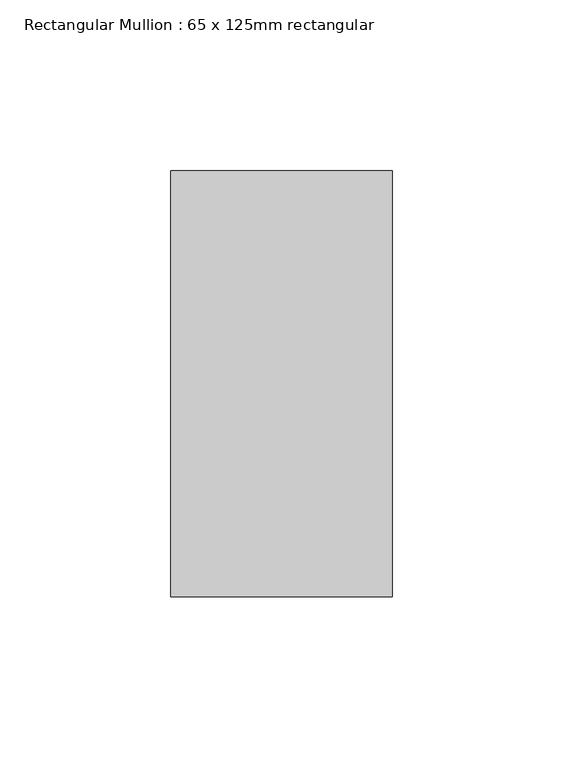
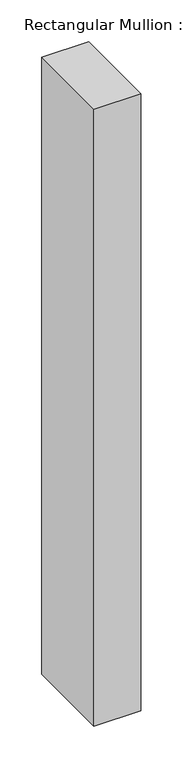
"""IFC4 building model written with IfcOpenShell, lengths in millimetres: member geometry, Rectangular Mullion : 65 x 125mm rectangular."""

from ifc_helpers import new_model, si_unit, frame, origin, place, context, project, spatial, polyline, outline, extrude, source, transform, mapped, element, save


def rectangular_mullion_65_x_125mm_rectangular_fcec82ed(model_context):
    return source(origin(), model_context, "Body", "SweptSolid", [
        extrude(outline(polyline([(0.0, 62.5), (0.0, -62.5), (-65.0, -62.5), (-65.0, 62.5), (0.0, 62.5)])), frame((0.0, 0.0, -902.5), z_axis=(0.0, 0.0, 1.0), x_axis=(1.0, 0.0, 0.0)), (0.0, 0.0, 1.0), 902.5),
    ])


if __name__ == "__main__":
    model = new_model("IFC4")
    model_context = context("Model", 3, world=origin())
    ifc_project = project(units=[si_unit("LENGTHUNIT", "METRE", prefix="MILLI")], contexts=[model_context])
    site = spatial("IfcSite", under=ifc_project)
    building = spatial("IfcBuilding", under=site)
    placement = place(None, origin())
    rectangular_mullion_65_x_125mm_rectangular_shape = rectangular_mullion_65_x_125mm_rectangular_fcec82ed(model_context)
    element("IfcMember", 1, ObjectType="Rectangular Mullion : 65 x 125mm rectangular", at=placement, inside=building, context=model_context, shape_type="MappedRepresentation", body=[
        mapped(rectangular_mullion_65_x_125mm_rectangular_shape, transform((0.0, 0.0, 0.0), x_axis=(1.0, 0.0, 0.0), y_axis=(0.0, 1.0, 0.0), z_axis=(0.0, 0.0, 1.0))),
    ])
    save(model, "model.ifc")

# Revit data of these elements
# Type "Rectangular Mullion : 65 x 125mm rectangular"
#   built-in parameter 1007304 = 0.410105 (stored number, unit not read)
#   built-in parameter 1007301 = 0.106627 (stored number, unit not read)
#   built-in parameter 1007300 = 0.106627 (stored number, unit not read)
# Element 1 (IfcMember, "Rectangular Mullion : 65 x 125mm rectangular")
#   Materials on its faces: "Aluminum"
# Materials
#   "Aluminum": class "Metal", colour RGB 244 245 246, transparency 0, Description = "Aluminum 6061", Cost = 0
